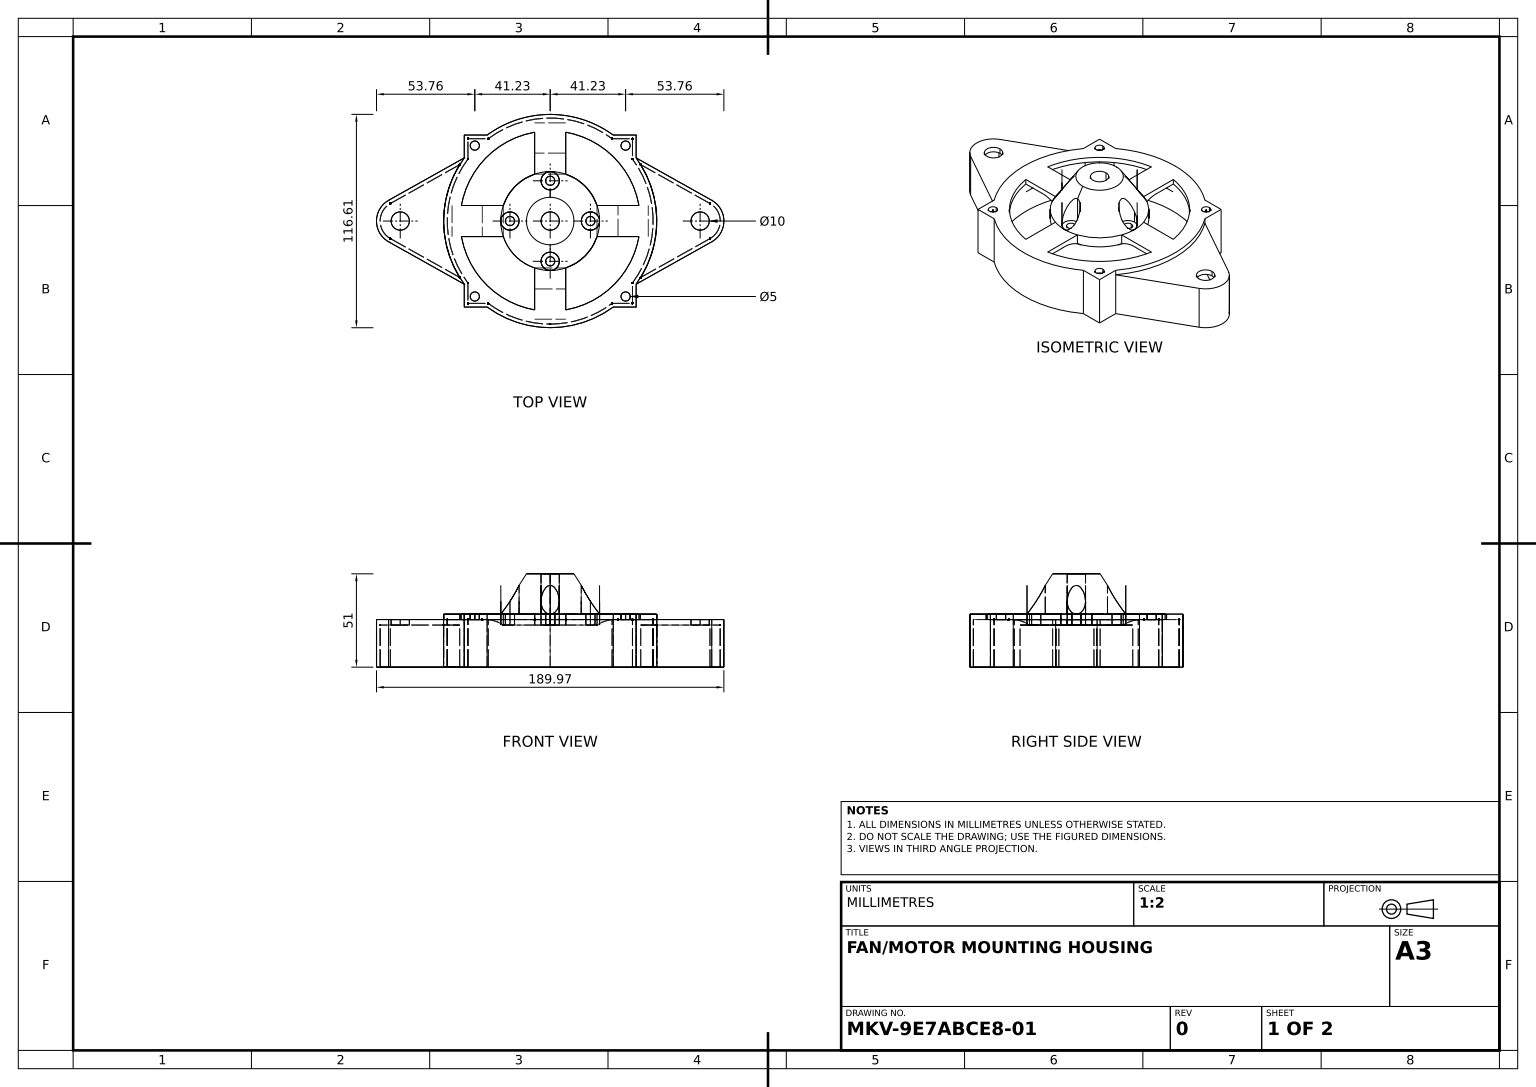
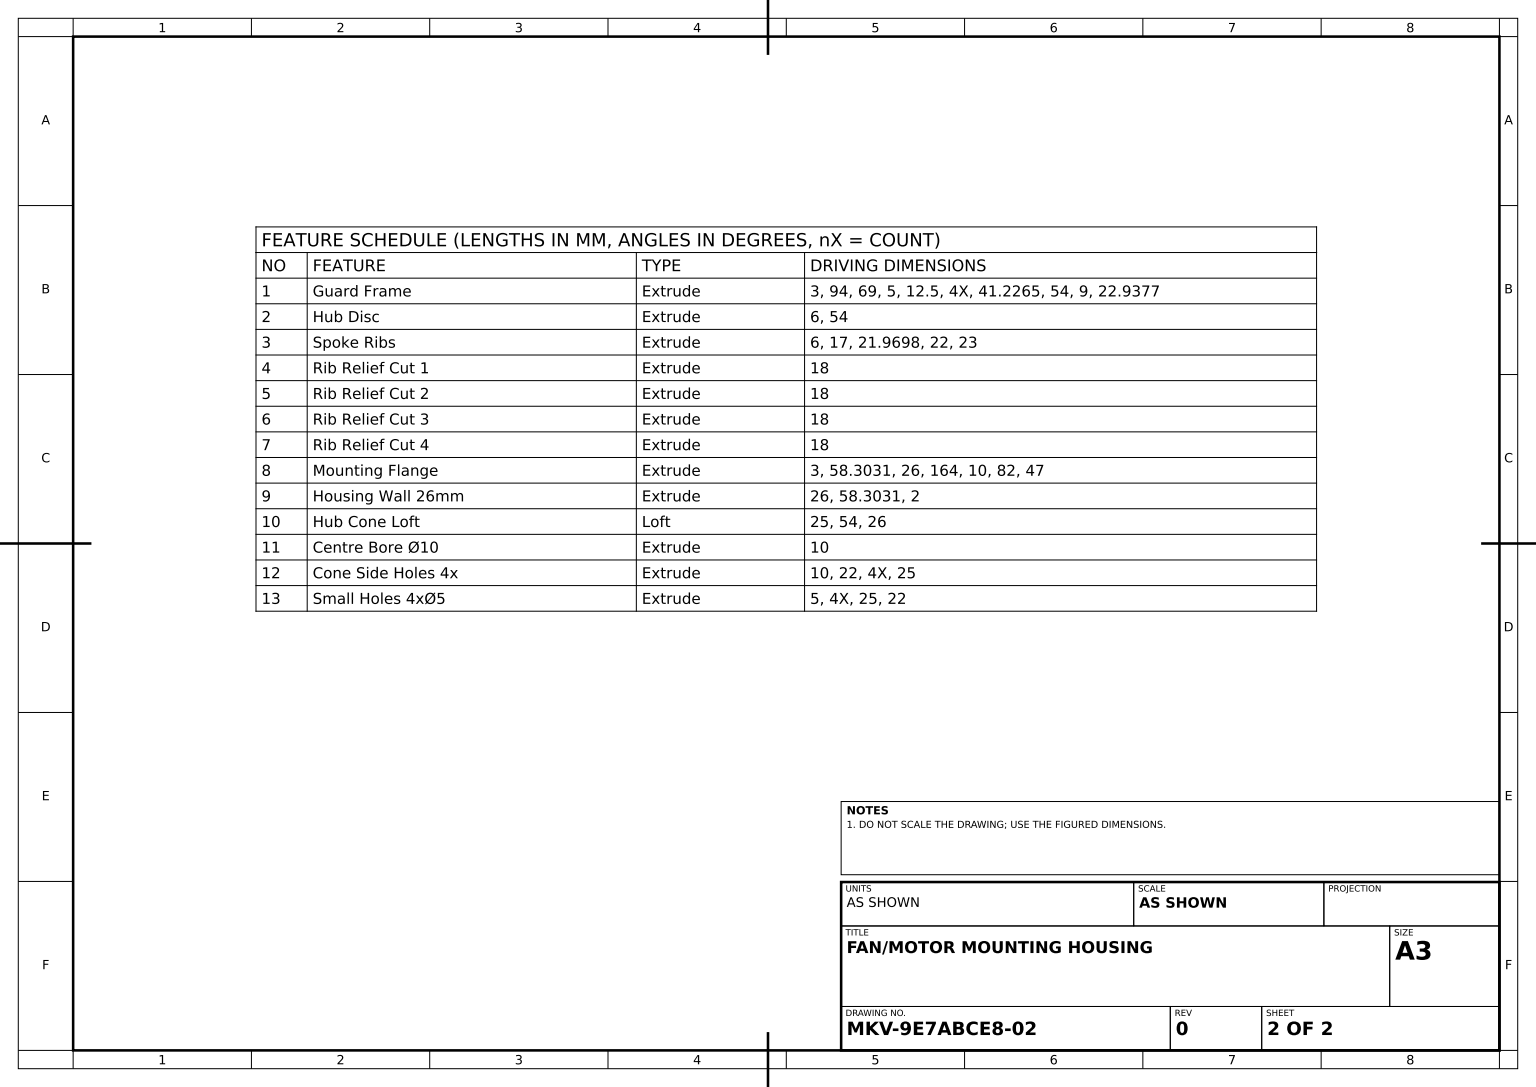
from build123d import *
from build123d.topology import SkipClean

# Parameters (mm, degrees)
GUARD_FRAME_SKETCH_R     = 2.5
GUARD_FRAME_SKETCH_R_2   = 27
GUARD_FRAME_DEPTH        = 3
HUB_START                = -6
HUB_DISC_SKETCH_R        = 27
HUB_DISC_DEPTH           = 6
SPOKE_RIBS_SKETCH_W      = 21.96978335
SPOKE_RIBS_SKETCH_H      = 17
SPOKE_RIBS_SKETCH_W_2    = 17
SPOKE_RIBS_SKETCH_H_2    = 22
SPOKE_RIBS_SKETCH_W_3    = 23
SPOKE_RIBS_DEPTH         = 6
RIB_RELIEF_CUT_1_DEPTH   = 17
RIB_RELIEF_CUT_2_DEPTH   = 17
RIB_RELIEF_CUT_3_DEPTH   = 17
RIB_RELIEF_CUT_4_DEPTH   = 17
MOUNTING_FLANGE_SKETCH_R = 5
MOUNTING_FLANGE_DEPTH    = 3
MOUNTING_FLANGE_2_DEPTH  = 3
HOUSING_START            = 26
HOUSING_WALL_26MM_DEPTH  = 26
CONE_BASE_CIRCLE_R       = 27
CONE_TOP_CIRCLE_R        = 13
CENTRE_BORE_SKETCH_R     = 5
CENTRE_BORE_10_DEPTH     = 123.577526488
CONE_SIDE_HOLES_SKETCH_R = 5
CONE_SIDE_HOLES_4X_DEPTH = 22
SMALL_HOLES_SKETCH_R     = 2.5
SMALL_HOLES_4X_5_DEPTH   = 116.17486705


with BuildPart() as part:
    # Guard Frame Sketch → Guard Frame (new body)
    # profile 1 of 2: a face of its own
    with BuildSketch(Plane(origin=(0, 0, 0), x_dir=(1, 0, 0), z_dir=(0, 1, 0))):
        with BuildLine():
            Line((-47, -34.5), (-47, -47))
            Line((-47, -47), (-34.5, -47))
            ThreePointArc((-34.5, -47), (0, -58.303087397), (34.5, -47))
            Line((34.5, -47), (47, -47))
            Line((47, -47), (47, -34.5))
            ThreePointArc((47, -34.5), (58.303087397, 0), (47, 34.5))
            Line((47, 34.5), (47, 47))
            Line((47, 47), (34.5, 47))
            ThreePointArc((34.5, 47), (0, 58.303087397), (-34.5, 47))
            Line((-34.5, 47), (-47, 47))
            Line((-47, 47), (-47, 34.5))
            ThreePointArc((-47, 34.5), (-58.303087397, 0), (-47, -34.5))
        make_face()
        with Locations(Location((-41.226508462, -41.226508462, 0), (0, 0, 270))):
            Circle(GUARD_FRAME_SKETCH_R, mode=Mode.SUBTRACT)
        with Locations(Location((41.226508462, -41.226508462, 0), (0, 0, 270))):
            Circle(GUARD_FRAME_SKETCH_R, mode=Mode.SUBTRACT)
        with Locations(Location((-41.226508462, 41.226508462, 0), (0, 0, 270))):
            Circle(GUARD_FRAME_SKETCH_R, mode=Mode.SUBTRACT)
        with BuildLine():
            Line((-8.5, 48.564847646), (-8.5, 25.627134057))
            ThreePointArc((-8.5, 25.627134057), (0, 27), (8.5, 25.627134057))
            Line((8.5, 25.627134057), (8.5, 48.564847646))
            ThreePointArc((8.5, 48.564847646), (34.862547432, 34.862547432), (48.564847646, 8.5))
            Line((48.564847646, 8.5), (25.627134057, 8.5))
            ThreePointArc((25.627134057, 8.5), (26.6545739, 4.305077261), (27, 0))
            ThreePointArc((27, 0), (26.6545739, -4.305077261), (25.627134057, -8.5))
            Line((25.627134057, -8.5), (48.564847646, -8.5))
            ThreePointArc((48.564847646, -8.5), (34.862547432, -34.862547432), (8.5, -48.564847646))
            Line((8.5, -48.564847646), (8.5, -25.627134057))
            ThreePointArc((8.5, -25.627134057), (0, -27), (-8.5, -25.627134057))
            Line((-8.5, -25.627134057), (-8.5, -48.564847646))
            ThreePointArc((-8.5, -48.564847646), (-34.862547432, -34.862547432), (-48.564847646, -8.5))
            Line((-48.564847646, -8.5), (-25.627134057, -8.5))
            ThreePointArc((-25.627134057, -8.5), (-27, 0), (-25.627134057, 8.5))
            Line((-25.627134057, 8.5), (-48.564847646, 8.5))
            ThreePointArc((-48.564847646, 8.5), (-34.862547432, 34.862547432), (-8.5, 48.564847646))
        make_face(mode=Mode.SUBTRACT)
        with Locations(Location((41.226508462, 41.226508462, 0), (0, 0, 270))):
            Circle(GUARD_FRAME_SKETCH_R, mode=Mode.SUBTRACT)
    # profile 2 of 2: a face of its own
    with BuildSketch(Plane(origin=(0, 0, 0), x_dir=(1, 0, 0), z_dir=(0, 1, 0))):
        Circle(GUARD_FRAME_SKETCH_R_2)
    extrude(amount=GUARD_FRAME_DEPTH)

    # Hub Disc Sketch → Hub Disc (add)
    with SkipClean():  # the faces are left unmerged after this step: merging them gives an invalid solid
        with BuildSketch(Plane(origin=(0, 3, 0), x_dir=(1, 0, 0), z_dir=(0, 1, 0)).offset(HUB_START)):
            with Locations(Location((0, 0, 0), (0, 0, 71.650365301))):
                Circle(HUB_DISC_SKETCH_R)
        extrude(amount=HUB_DISC_DEPTH)

    # Spoke Ribs Sketch → Spoke Ribs (add)
    with BuildSketch(Plane(origin=(0, 3, 0), x_dir=(1, 0, 0), z_dir=(0, 1, 0))):
        with Locations((-26.111099177, 0)):
            Rectangle(SPOKE_RIBS_SKETCH_W, SPOKE_RIBS_SKETCH_H)
        with Locations((0, 26.095990852)):
            Rectangle(SPOKE_RIBS_SKETCH_W_2, SPOKE_RIBS_SKETCH_H_2)
        with Locations((25.595990852, 0)):
            Rectangle(SPOKE_RIBS_SKETCH_W_3, SPOKE_RIBS_SKETCH_H)
        with Locations((0, -26.095990852)):
            Rectangle(SPOKE_RIBS_SKETCH_W_2, SPOKE_RIBS_SKETCH_H_2)
    extrude(amount=-SPOKE_RIBS_DEPTH)

    # Rib Relief Cut 1 Sketch → Rib Relief Cut 1 (cut)
    with BuildSketch(Plane.XY.offset(8.5)):
        with BuildLine():
            Line((-37.095990852, 0), (-37.095990852, -3))
            Line((-37.095990852, -3), (-25.627134057, -3))
            ThreePointArc((-25.627134057, -3), (-31.107503937, -0.528746416), (-37.095990852, 0))
        make_face()
    extrude(amount=-RIB_RELIEF_CUT_1_DEPTH, mode=Mode.SUBTRACT)

    # Rib Relief Cut 2 Sketch → Rib Relief Cut 2 (cut)
    with BuildSketch(Plane.ZY.offset(8.5)):
        with BuildLine():
            Line((-37.095990852, 0), (-37.095990852, -3))
            Line((-37.095990852, -3), (-25.627134057, -3))
            ThreePointArc((-25.627134057, -3), (-31.107503937, -0.528746416), (-37.095990852, 0))
        make_face()
    extrude(amount=-RIB_RELIEF_CUT_2_DEPTH, mode=Mode.SUBTRACT)

    # Rib Relief Cut 3 Sketch → Rib Relief Cut 3 (cut)
    with BuildSketch(Plane(origin=(0, 0, -8.5), x_dir=(-1, 0, 0), z_dir=(0, 0, -1))):
        with BuildLine():
            Line((-37.095990852, 0), (-37.095990852, -3))
            Line((-37.095990852, -3), (-25.627134057, -3))
            ThreePointArc((-25.627134057, -3), (-31.107503937, -0.528746416), (-37.095990852, 0))
        make_face()
    extrude(amount=-RIB_RELIEF_CUT_3_DEPTH, mode=Mode.SUBTRACT)

    # Rib Relief Cut 4 Sketch → Rib Relief Cut 4 (cut)
    with BuildSketch(Plane(origin=(8.5, 0, 0), x_dir=(0, 0, -1), z_dir=(1, 0, 0))):
        with BuildLine():
            Line((-37.095990852, 0), (-37.095990852, -3))
            Line((-37.095990852, -3), (-25.627134057, -3))
            ThreePointArc((-25.627134057, -3), (-31.107503937, -0.528746416), (-37.095990852, 0))
        make_face()
    extrude(amount=-RIB_RELIEF_CUT_4_DEPTH, mode=Mode.SUBTRACT)



with BuildPart() as body_2:
    # Mounting Flange Sketch → Mounting Flange (new body)
    with BuildSketch(Plane.XZ):
        with BuildLine():
            Line((-47, 34.5), (-88.351925079, 11.342532689))
            ThreePointArc((-88.351925079, 11.342532689), (-95, 0), (-88.351925079, -11.342532689))
            Line((-88.351925079, -11.342532689), (-47, -34.5))
            ThreePointArc((-47, -34.5), (-58.303087397, 0), (-47, 34.5))
        make_face()
        with Locations(Location((-82, 0, 0), (0, 0, 270))):
            Circle(MOUNTING_FLANGE_SKETCH_R, mode=Mode.SUBTRACT)
    extrude(amount=MOUNTING_FLANGE_DEPTH)


with BuildPart() as body_3:
    # Mounting Flange Sketch → Mounting Flange 2 (new body)
    with BuildSketch(Plane.XZ):
        with BuildLine():
            Line((47, 34.5), (88.351925079, 11.342532689))
            ThreePointArc((88.351925079, 11.342532689), (95, 0), (88.351925079, -11.342532689))
            Line((88.351925079, -11.342532689), (47, -34.5))
            ThreePointArc((47, -34.5), (58.303087397, 0), (47, 34.5))
        make_face()
        with Locations(Location((82, 0, 0), (0, 0, 270))):
            Circle(MOUNTING_FLANGE_SKETCH_R, mode=Mode.SUBTRACT)
    extrude(amount=MOUNTING_FLANGE_2_DEPTH)


with BuildPart() as part_1:
    add(part.part)

    add(body_2.part)  # Housing Wall 26mm merges body 2

    add(body_3.part)  # Housing Wall 26mm merges body 3
    # Housing Wall Sketch → Housing Wall 26mm (add)
    # profile 1 of 3: a face of its own
    with BuildSketch(Plane.XZ.offset(HOUSING_START)):
        with BuildLine():
            ThreePointArc((-34.5, -47), (0, -58.303087397), (34.5, -47))
            Line((34.5, -47), (47, -47))
            Line((47, -47), (47, -34.5))
            ThreePointArc((47, -34.5), (58.303087397, 0), (47, 34.5))
            Line((47, 34.5), (47, 47))
            Line((47, 47), (34.5, 47))
            ThreePointArc((34.5, 47), (0, 58.303087397), (-34.5, 47))
            Line((-34.5, 47), (-47, 47))
            Line((-47, 47), (-47, 34.5))
            ThreePointArc((-47, 34.5), (-58.303087397, 0), (-47, -34.5))
            Line((-47, -34.5), (-47, -47))
            Line((-47, -47), (-34.5, -47))
        make_face()
        with BuildLine():
            ThreePointArc((-33.838404963, -45), (0, -56.303087397), (33.838404963, -45))
            Line((33.838404963, -45), (45, -45))
            Line((45, -45), (45, -33.838404963))
            ThreePointArc((45, -33.838404963), (56.303087397, 0), (45, 33.838404963))
            Line((45, 33.838404963), (45, 45))
            Line((45, 45), (33.838404963, 45))
            ThreePointArc((33.838404963, 45), (0, 56.303087397), (-33.838404963, 45))
            Line((-33.838404963, 45), (-45, 45))
            Line((-45, 45), (-45, 33.838404963))
            ThreePointArc((-45, 33.838404963), (-56.303087397, 0), (-45, -33.838404963))
            Line((-45, -33.838404963), (-45, -45))
            Line((-45, -45), (-33.838404963, -45))
        make_face(mode=Mode.SUBTRACT)
    # profile 2 of 3: a face of its own
    with BuildSketch(Plane.XZ.offset(HOUSING_START)):
        with BuildLine():
            Line((-47, 34.5), (-88.351925079, 11.342532689))
            ThreePointArc((-88.351925079, 11.342532689), (-95, 0), (-88.351925079, -11.342532689))
            Line((-88.351925079, -11.342532689), (-47, -34.5))
            ThreePointArc((-47, -34.5), (-48.284390978, -32.678243341), (-49.498207875, -30.808723069))
            Line((-49.498207875, -30.808723069), (-87.374705836, -9.59752766))
            ThreePointArc((-87.374705836, -9.59752766), (-93, 0), (-87.374705836, 9.59752766))
            Line((-87.374705836, 9.59752766), (-49.498207875, 30.808723069))
            ThreePointArc((-49.498207875, 30.808723069), (-48.284390978, 32.678243341), (-47, 34.5))
        make_face()
    # profile 3 of 3: a face of its own
    with BuildSketch(Plane.XZ.offset(HOUSING_START)):
        with BuildLine():
            Line((88.351925079, 11.342532689), (47, 34.5))
            ThreePointArc((47, 34.5), (48.284390978, 32.678243341), (49.498207875, 30.808723069))
            Line((49.498207875, 30.808723069), (87.374705836, 9.59752766))
            ThreePointArc((87.374705836, 9.59752766), (93, 0), (87.374705836, -9.59752766))
            Line((87.374705836, -9.59752766), (49.498207875, -30.808723069))
            ThreePointArc((49.498207875, -30.808723069), (48.284390978, -32.678243341), (47, -34.5))
            Line((47, -34.5), (88.351925079, -11.342532689))
            ThreePointArc((88.351925079, -11.342532689), (95, 0), (88.351925079, 11.342532689))
        make_face()
    extrude(amount=-HOUSING_WALL_26MM_DEPTH)

    # Cone Base Circle → Hub Cone Loft section 0
    with BuildSketch(Plane(origin=(0, 3, 0), x_dir=(1, 0, 0), z_dir=(0, 1, 0))):
        Circle(CONE_BASE_CIRCLE_R)
    # Cone Top Circle → Hub Cone Loft section 1
    with BuildSketch(Plane(origin=(0, 25, 0), x_dir=(1, 0, 0), z_dir=(0, 1, 0))):
        Circle(CONE_TOP_CIRCLE_R)
    loft()

    # Centre Bore Sketch → Centre Bore Ø10 (cut, through all)
    with BuildSketch(Plane(origin=(0, 25, 0), x_dir=(1, 0, 0), z_dir=(0, 1, 0))):
        with Locations(Location((0, 0, 0), (0, 0, 270))):
            Circle(CENTRE_BORE_SKETCH_R)
    extrude(amount=-CENTRE_BORE_10_DEPTH, mode=Mode.SUBTRACT)

    # Cone Side Holes Sketch → Cone Side Holes 4x (cut)
    with SkipClean():  # the faces are left unmerged after this step: merging them gives an invalid solid
        with BuildSketch(Plane(origin=(0, 25, 0), x_dir=(1, 0, 0), z_dir=(0, 1, 0))):
            with Locations((0, 22)):
                Circle(CONE_SIDE_HOLES_SKETCH_R)
            with Locations((22, 0)):
                Circle(CONE_SIDE_HOLES_SKETCH_R)
            with Locations((0, -22)):
                Circle(CONE_SIDE_HOLES_SKETCH_R)
            with Locations((-22, 0)):
                Circle(CONE_SIDE_HOLES_SKETCH_R)
        extrude(amount=-CONE_SIDE_HOLES_4X_DEPTH, mode=Mode.SUBTRACT)

    # Small Holes Sketch → Small Holes 4xØ5 (cut, through all)
    with SkipClean():  # the faces are left unmerged after this step: merging them gives an invalid solid
        with BuildSketch(Plane(origin=(0, 3, 0), x_dir=(1, 0, 0), z_dir=(0, 1, 0))):
            with Locations(Location((0, 22, 0), (0, 0, 270))):
                Circle(SMALL_HOLES_SKETCH_R)
            with Locations(Location((22, 0, 0), (0, 0, 270))):
                Circle(SMALL_HOLES_SKETCH_R)
            with Locations(Location((0, -22, 0), (0, 0, 270))):
                Circle(SMALL_HOLES_SKETCH_R)
            with Locations(Location((-22, 0, 0), (0, 0, 270))):
                Circle(SMALL_HOLES_SKETCH_R)
        extrude(amount=-SMALL_HOLES_4X_5_DEPTH, mode=Mode.SUBTRACT)


solid = part_1.part
